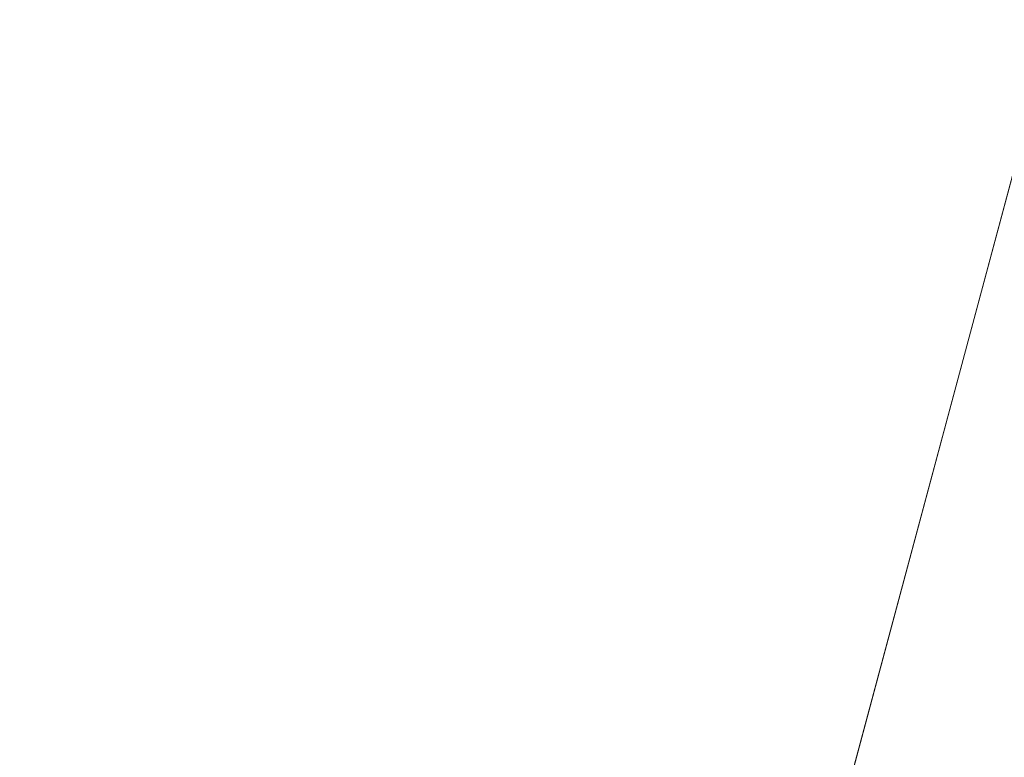
# Model space of a CAD drawing. Units: inches. Extents: x 375 to 1122, y 27 to 1069.
# Tile 56 of 155: x 732.625 to 734.823, y 304.063 to 305.711. Entities that reach past the tile are written whole.
import ezdxf

# ---------------------------------------------------------------- set-up
doc = ezdxf.new("R2010")
doc.units = ezdxf.units.IN
doc.layers.add('A-ANNO-DIMS', color=2, linetype='Continuous', lineweight=18)
doc.layers.add('Furniture', color=30, linetype='Continuous', lineweight=18)
doc.styles.get("Standard").update_dxf_attribs({"font": 'arial.ttf'})
doc.dimstyles.new('ISO-25', dxfattribs={"dimtxt": 12, "dimasz": 2.5, "dimexe": 1.5, "dimexo": 1.5, "dimtad": 1, "dimdec": 1, "dimlunit": 3, "dimtxsty": 'Standard', "dimblk": 'ARCHTICK', "dimcen": 2.5, "dimadec": 0, "dimazin": 0, "dimtfac": 1, "dimtdec": 1, "dimtmove": 0, "dimatfit": 3, "dimfxl": 1.5, "dimfxlon": 1, "dimarcsym": 0})

# ---------------------------------------------------------------- blocks, each defined once
blk = doc.blocks.new('A$C403C54AD')
at = {"linetype": 'ByBlock', "invisible_edges": 5}
for points in [[(1.027872, 1.280047, -0.037345), (1.010941, 1.250721, -0.02811), (1.080205, 1.232162, -0.02811), (1.080205, 1.266024, -0.037345)], [(1.010941, 1.250721, -0.023492), (1.020176, 1.266717, -0.023492), (1.080205, 1.250632, -0.023492), (1.080205, 1.232162, -0.023492)]]:
    blk.add_3dface(points, dxfattribs=at)
at = {"linetype": 'ByBlock'}
blk.add_3dface([(1.010941, 1.250721, -0.02811), (1.010941, 1.250721, -0.023492), (1.080205, 1.232162, -0.023492), (1.080205, 1.232162, -0.02811)], dxfattribs=at)
blk = doc.blocks.new('_ArchTick')
at = {"color": 0, "linetype": 'ByBlock', "const_width": 0.15}
blk.add_lwpolyline([(-0.5, -0.5), (0.5, 0.5)], dxfattribs=at)
blk = doc.blocks.new('*D94')
at = {"layer": 'A-ANNO-DIMS', "color": 0, "lineweight": -2, "transparency": 16777216}
for p, q in [((734.0073, 117.5277), (734.0073, 114.5277)), ((773.0073, 117.5277), (773.0073, 114.5277)), ((734.0073, 116.0277), (773.0073, 116.0277))]:
    blk.add_line(p, q, dxfattribs=at)
at = {"layer": 'Defpoints', "color": 0, "transparency": 16777216}
for p in [(734.0073, 667.5277), (773.0073, 667.5277), (773.0073, 116.0277)]:
    blk.add_point(p, dxfattribs=at)
at = {"layer": 'A-ANNO-DIMS', "color": 0, "lineweight": -2, "transparency": 16777216, "xscale": 2.5, "yscale": 2.5, "zscale": 2.5, "rotation": 180}
blk.add_blockref('_ArchTick', (734.0073, 116.0277), dxfattribs=at)
at = {"layer": 'A-ANNO-DIMS', "color": 0, "lineweight": -2, "transparency": 16777216, "xscale": 2.5, "yscale": 2.5, "zscale": 2.5}
blk.add_blockref('_ArchTick', (773.0073, 116.0277), dxfattribs=at)
at = {"layer": 'A-ANNO-DIMS', "color": 0, "transparency": 16777216, "insert": (753.5073, 122.7837), "char_height": 12, "attachment_point": 5}
blk.add_mtext('3\'-3"', dxfattribs=at)

msp = doc.modelspace()

# ---------------------------------------------------------------- block references
at = {"layer": 'Furniture', "xscale": 39.9918517141215, "yscale": 39.9918517141215, "zscale": 39.9918517141215, "rotation": 270}
msp.add_blockref('A$C403C54AD', (684.9549, 346.2875, 0.024), dxfattribs=at)

# ---------------------------------------------------------------- dimensions: what is measured, and where the dimension line sits
at = {"layer": 'A-ANNO-DIMS'}
dim = msp.add_linear_dim(base=(773.0073, 116.0277), p1=(734.0073, 667.5277), p2=(773.0073, 667.5277), dimstyle='ISO-25', override={"dimdec": 1, "dimlfac": 1, "dimrnd": 0, "dimzin": 1, "dimdsep": 46, "dimlunit": 4, "dimfrac": 2}, dxfattribs=at)
dim.commit()
dim.dimension.update_dxf_attribs({"geometry": '*D94', "text_midpoint": (753.5073, 122.7837)})

doc.saveas('drawing.dxf')
